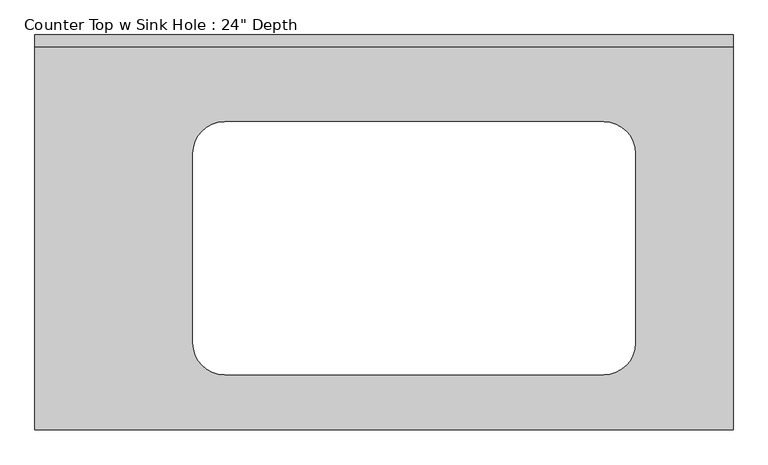
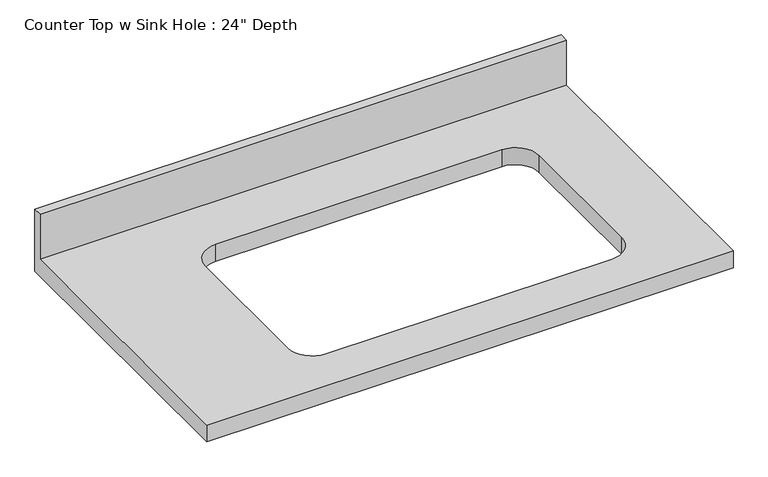
"""IFC4 building model written with IfcOpenShell, lengths in millimetres: furniture geometry."""

from ifc_helpers import new_model, si_unit, frame, origin, place, context, project, spatial, polyline, circle_curve, source, transform, mapped, element, save
from ifc_brep_helpers import plane_surface, revolved_surface, advanced_brep


def furniture_53e129a0(model_context):
    return source(origin(), model_context, "Body", "AdvancedBrep", [
        advanced_brep(
        [(-1200.4622951, -635.0, 914.4), (-78.1397312, -635.0, 914.4), (-78.1397312, -19.05, 914.4), (-1200.4622951, -19.05, 914.4), (-895.6622951, -139.7, 914.4), (-286.0622951, -139.7, 914.4), (-235.2622951, -190.5, 914.4), (-235.2622951, -495.3, 914.4), (-286.0622951, -546.1, 914.4), (-895.6622951, -546.1, 914.4), (-946.4622951, -495.3, 914.4), (-946.4622951, -190.5, 914.4), (-78.1397312, 0.0, 876.3), (-78.1397312, -635.0, 876.3), (-1200.4622951, -635.0, 876.3), (-1200.4622951, 0.0, 876.3), (-286.0622951, -139.7, 876.3), (-895.6622951, -139.7, 876.3), (-946.4622951, -190.5, 876.3), (-946.4622951, -495.3, 876.3), (-895.6622951, -546.1, 876.3), (-286.0622951, -546.1, 876.3), (-235.2622951, -495.3, 876.3), (-235.2622951, -190.5, 876.3), (-1200.4622951, 0.0, 1016.0), (-78.1397312, 0.0, 1016.0), (-1200.4622951, -19.05, 1016.0), (-78.1397312, -19.05, 1016.0)],
        [
            (0, 1),
            (1, 2),
            (2, 3),
            (3, 0),
            (4, 5),
            (5, 6, circle_curve(frame((-286.0622951, -190.5, 914.4), z_axis=(0.0, 0.0, -1.0), x_axis=(1.0, 0.0, 0.0)), 50.8)),
            (6, 7),
            (7, 8, circle_curve(frame((-286.0622951, -495.3, 914.4), z_axis=(0.0, 0.0, -1.0), x_axis=(1.0, 0.0, 0.0)), 50.8)),
            (8, 9),
            (9, 10, circle_curve(frame((-895.6622951, -495.3, 914.4), z_axis=(0.0, 0.0, -1.0), x_axis=(1.0, 0.0, 0.0)), 50.8)),
            (10, 11),
            (11, 4, circle_curve(frame((-895.6622951, -190.5, 914.4), z_axis=(0.0, 0.0, -1.0), x_axis=(1.0, 0.0, 0.0)), 50.8)),
            (12, 13),
            (13, 14),
            (14, 15),
            (15, 12),
            (16, 17),
            (17, 18, circle_curve(frame((-895.6622951, -190.5, 876.3), z_axis=(0.0, 0.0, 1.0), x_axis=(1.0, 0.0, 0.0)), 50.8)),
            (18, 19),
            (19, 20, circle_curve(frame((-895.6622951, -495.3, 876.3), z_axis=(0.0, 0.0, 1.0), x_axis=(1.0, 0.0, 0.0)), 50.8)),
            (20, 21),
            (21, 22, circle_curve(frame((-286.0622951, -495.3, 876.3), z_axis=(0.0, 0.0, 1.0), x_axis=(1.0, 0.0, 0.0)), 50.8)),
            (22, 23),
            (23, 16, circle_curve(frame((-286.0622951, -190.5, 876.3), z_axis=(0.0, 0.0, 1.0), x_axis=(1.0, 0.0, 0.0)), 50.8)),
            (15, 24),
            (24, 25),
            (25, 12),
            (14, 0),
            (3, 26),
            (26, 24),
            (13, 1),
            (25, 27),
            (27, 2),
            (26, 27),
            (4, 17),
            (16, 5),
            (11, 18),
            (10, 19),
            (9, 20),
            (8, 21),
            (7, 22),
            (6, 23),
        ],
        [
            plane_surface(frame((-1200.4622951, 0.0, 914.4), z_axis=(0.0, 0.0, 1.0), x_axis=(-1.0, 0.0, 0.0))),
            plane_surface(frame((-1200.4622951, 0.0, 876.3), z_axis=(0.0, 0.0, -1.0), x_axis=(1.0, 0.0, 0.0))),
            plane_surface(frame((-78.1397312, 0.0, 914.4), z_axis=(0.0, 1.0, 0.0), x_axis=(0.0, 0.0, -1.0))),
            plane_surface(frame((-1200.4622951, 0.0, 914.4), z_axis=(-1.0, 0.0, 0.0), x_axis=(0.0, 0.0, -1.0))),
            plane_surface(frame((-1200.4622951, -635.0, 914.4), z_axis=(0.0, -1.0, 0.0), x_axis=(0.0, 0.0, -1.0))),
            plane_surface(frame((-78.1397312, -635.0, 914.4), z_axis=(1.0, 0.0, 0.0), x_axis=(0.0, 0.0, -1.0))),
            plane_surface(frame((-1200.4622951, 0.0, 1016.0), z_axis=(0.0, 0.0, 1.0), x_axis=(0.0, -1.0, 0.0))),
            plane_surface(frame((-1200.4622951, -19.05, 1016.0), z_axis=(0.0, -1.0, 0.0), x_axis=(0.0, 0.0, -1.0))),
            plane_surface(frame((-286.0622951, -139.7, 914.4), z_axis=(0.0, -1.0, 0.0), x_axis=(0.0, 0.0, -1.0))),
            revolved_surface(polyline([(-844.8622951000001, -190.5, 914.4), (-844.8622951000001, -190.5, 876.3)]), (-895.6622951, -190.5, 876.3), (0.0, 0.0, 1.0)),
            plane_surface(frame((-946.4622951, -190.5, 914.4), z_axis=(1.0, 0.0, 0.0), x_axis=(0.0, 0.0, -1.0))),
            revolved_surface(polyline([(-844.8622951000001, -495.3, 914.4), (-844.8622951000001, -495.3, 876.3)]), (-895.6622951, -495.3, 876.3), (0.0, 0.0, 1.0)),
            plane_surface(frame((-895.6622951, -546.1, 914.4), z_axis=(0.0, 1.0, 0.0), x_axis=(0.0, 0.0, -1.0))),
            revolved_surface(polyline([(-235.26229509999996, -495.3, 914.4), (-235.26229509999996, -495.3, 876.3)]), (-286.0622951, -495.3, 876.3), (0.0, 0.0, 1.0)),
            plane_surface(frame((-235.2622951, -495.3, 914.4), z_axis=(-1.0, 0.0, 0.0), x_axis=(0.0, 0.0, -1.0))),
            revolved_surface(polyline([(-235.26229509999996, -190.5, 914.4), (-235.26229509999996, -190.5, 876.3)]), (-286.0622951, -190.5, 876.3), (0.0, 0.0, 1.0)),
        ],
        [
            (0, [[1, 2, 3, 4], [5, 6, 7, 8, 9, 10, 11, 12]]),
            (1, [[13, 14, 15, 16], [17, 18, 19, 20, 21, 22, 23, 24]]),
            (2, [[-16, 25, 26, 27]]),
            (3, [[-15, 28, -4, 29, 30, -25]]),
            (4, [[-1, -28, -14, 31]]),
            (5, [[-13, -27, 32, 33, -2, -31]]),
            (6, [[-30, 34, -32, -26]]),
            (7, [[-34, -29, -3, -33]]),
            (8, [[35, -17, 36, -5]]),
            (9, [[-35, -12, 37, -18]]),
            (10, [[-37, -11, 38, -19]]),
            (11, [[-38, -10, 39, -20]]),
            (12, [[-39, -9, 40, -21]]),
            (13, [[-40, -8, 41, -22]]),
            (14, [[-41, -7, 42, -23]]),
            (15, [[-36, -24, -42, -6]]),
        ],
    ),
    ])


if __name__ == "__main__":
    model = new_model("IFC4")
    model_context = context("Model", 3, world=origin())
    ifc_project = project(units=[si_unit("LENGTHUNIT", "METRE", prefix="MILLI")], contexts=[model_context])
    site = spatial("IfcSite", under=ifc_project)
    building = spatial("IfcBuilding", under=site)
    placement = place(None, origin())
    furniture_shape = furniture_53e129a0(model_context)
    element("IfcFurniture", 1, ObjectType="Counter Top w Sink Hole : 24\" Depth", at=placement, inside=building, context=model_context, shape_type="MappedRepresentation", body=[
        mapped(furniture_shape, transform((0.0, 0.0, 0.0), x_axis=(1.0, 0.0, 0.0), y_axis=(0.0, 1.0, 0.0), z_axis=(0.0, 0.0, 1.0))),
    ])
    save(model, "model.ifc")

# Revit data of these elements
# Type "Counter Top w Sink Hole : 24\" Depth"
#   Assembly Code = "C1030400"
#   Counter Thickness = 0' - 1 1/2"
#   Depth = 2' - 1"
#   Height = 3' - 0"
#   Length [instance default] = 8' - 0"
#   Sink Location [instance default] = 2' - 0"
#   Sink Location To Wall [instance default] = 0' - 6"
#   Sink Opening Depth [instance default] = 1' - 3"
#   Sink Opening Width [instance default] = 2' - 3"
#   Counter Top Material = none
#   Default Elevation = 0
# Element 1 (IfcFurniture, "Counter Top w Sink Hole : 24\" Depth")
#   Length = 3' - 8.18593"
#   Materials on its faces: "Counter Top"
# Materials
#   "Counter Top": class "Wood", colour RGB 226 177 128, transparency 0
